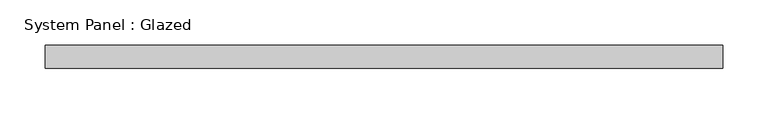
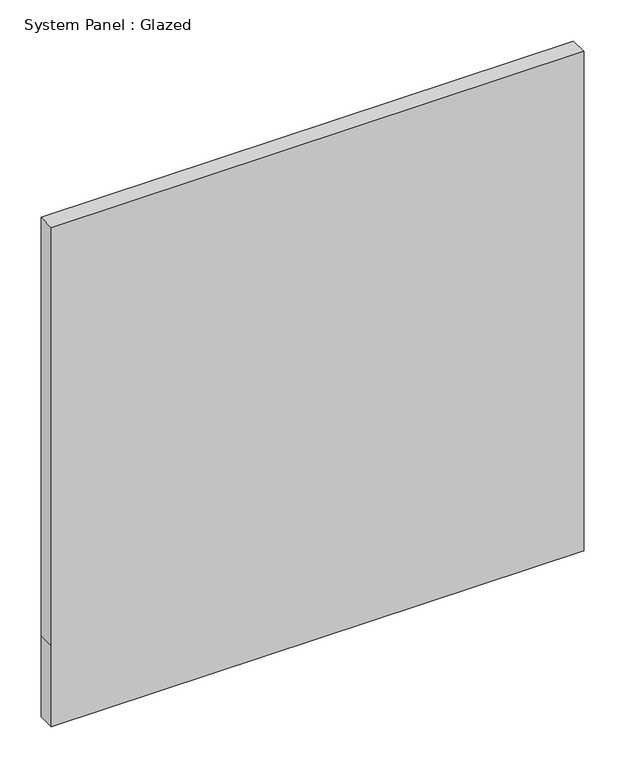
"""IFC4 building model written with IfcOpenShell, lengths in millimetres: plate geometry, System Panel : Glazed."""

from ifc_helpers import new_model, si_unit, frame, origin, place, context, project, spatial, polyline, outline, extrude, source, transform, mapped, element, save


def system_panel_glazed_02566968(model_context):
    return source(origin(), model_context, "Body", "SweptSolid", [
        extrude(outline(polyline([(0.0, -374.65), (0.0, 374.65), (120.65, 374.65), (742.6074877, 374.65), (742.6074877, -374.65), (120.65, -374.65), (0.0, -374.65)])), frame((0.0, 19.05, 0.0), z_axis=(0.0, 1.0, 0.0), x_axis=(0.0, 0.0, 1.0)), (0.0, 0.0, 1.0), 25.4),
    ])


if __name__ == "__main__":
    model = new_model("IFC4")
    model_context = context("Model", 3, world=origin())
    ifc_project = project(units=[si_unit("LENGTHUNIT", "METRE", prefix="MILLI")], contexts=[model_context])
    site = spatial("IfcSite", under=ifc_project)
    building = spatial("IfcBuilding", under=site)
    placement = place(None, origin())
    system_panel_glazed_shape = system_panel_glazed_02566968(model_context)
    element("IfcPlate", 1, ObjectType="System Panel : Glazed", at=placement, inside=building, context=model_context, shape_type="MappedRepresentation", body=[
        mapped(system_panel_glazed_shape, transform((0.0, 0.0, 0.0), x_axis=(1.0, 0.0, 0.0), y_axis=(0.0, 1.0, 0.0), z_axis=(0.0, 0.0, 1.0))),
    ])
    save(model, "model.ifc")

# Revit data of these elements
# Type "System Panel : Glazed"
#   Construction Type Id = "GSP4R"
#   Analytic Construction = "1/8 in Pilkington single glazing"
#   Visual Light Transmittance = 0.9
#   Solar Heat Gain Coefficient = 0.86
#   Heat Transfer Coefficient (U) = 1.18115 BTU/(h·ft²·°F)
#   Define Thermal Properties by = 1
# Element 1 (IfcPlate, "System Panel : Glazed")
#   Materials on its faces: "Glass"
# Materials
#   "Glass": class "Glass", colour RGB 0 128 192, transparency 0.75, Description = "Soda Lime Glass", Cost = 0
